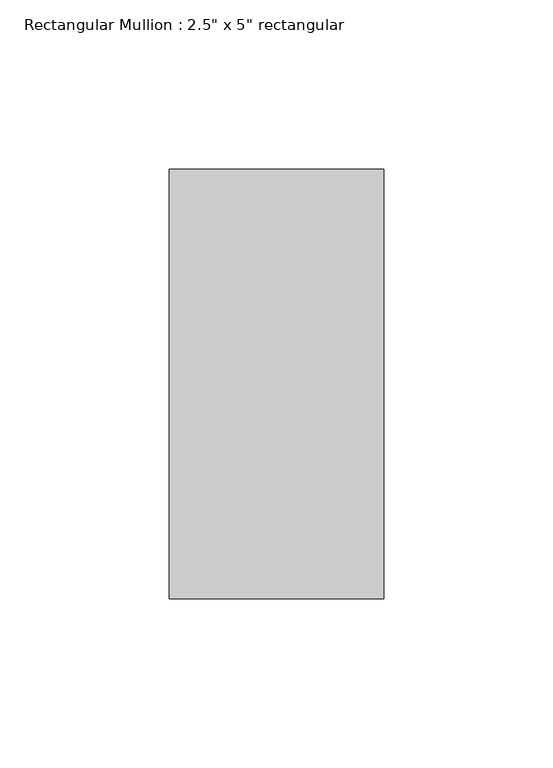
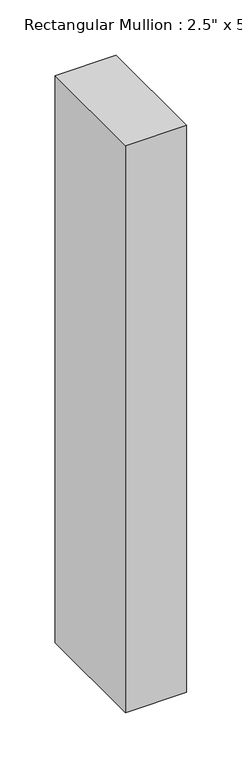
"""IFC4 building model written with IfcOpenShell, lengths in millimetres: member geometry."""

from ifc_helpers import new_model, si_unit, frame, origin, place, context, project, spatial, polyline, outline, extrude, source, transform, mapped, element, save


def member_b5a88f55(model_context):
    return source(origin(), model_context, "Body", "SweptSolid", [
        extrude(outline(polyline([(0.0, 63.5), (0.0, -63.5), (-63.5, -63.5), (-63.5, 63.5), (0.0, 63.5)])), frame((0.0, 0.0, -624.4166667), z_axis=(0.0, 0.0, 1.0), x_axis=(1.0, 0.0, 0.0)), (0.0, 0.0, 1.0), 624.4166667),
    ])


if __name__ == "__main__":
    model = new_model("IFC4")
    model_context = context("Model", 3, world=origin())
    ifc_project = project(units=[si_unit("LENGTHUNIT", "METRE", prefix="MILLI")], contexts=[model_context])
    site = spatial("IfcSite", under=ifc_project)
    building = spatial("IfcBuilding", under=site)
    placement = place(None, origin())
    member_shape = member_b5a88f55(model_context)
    element("IfcMember", 1, ObjectType="Rectangular Mullion : 2.5\" x 5\" rectangular", at=placement, inside=building, context=model_context, shape_type="MappedRepresentation", body=[
        mapped(member_shape, transform((0.0, 0.0, 0.0), x_axis=(1.0, 0.0, 0.0), y_axis=(0.0, 1.0, 0.0), z_axis=(0.0, 0.0, 1.0))),
    ])
    save(model, "model.ifc")

# Revit data of these elements
# Type "Rectangular Mullion : 2.5\" x 5\" rectangular"
#   built-in parameter 1007304 = 0.416667 (stored number, unit not read)
#   built-in parameter 1007301 = 0.104167 (stored number, unit not read)
#   built-in parameter 1007300 = 0.104167 (stored number, unit not read)
# Element 1 (IfcMember, "Rectangular Mullion : 2.5\" x 5\" rectangular")
#   Materials on its faces: "Aluminum"
# Materials
#   "Aluminum": class "Metal", colour RGB 247 247 247, transparency 0, Description = "Aluminum 6061", Cost = 0
